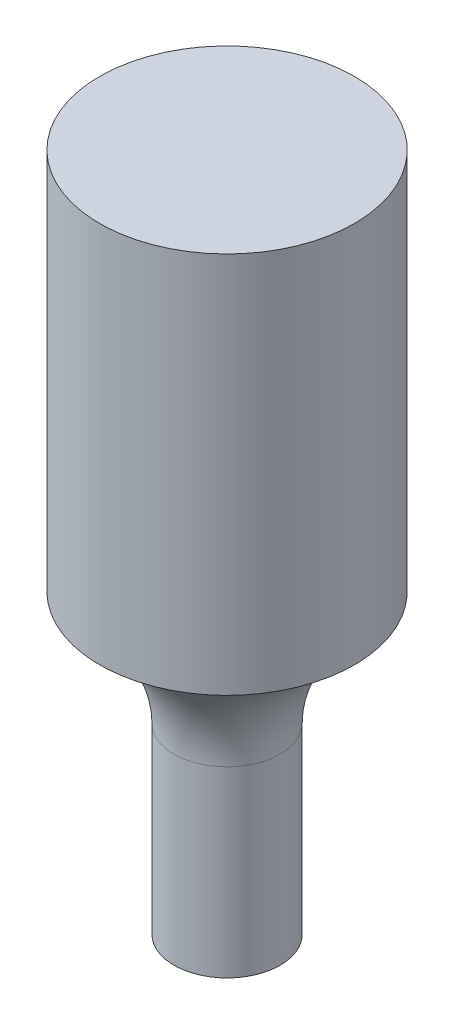
ISO-10303-21;
HEADER;
FILE_DESCRIPTION(('STEP AP214'),'2;1');
FILE_NAME('part.step','',(''),(''),'','','');
FILE_SCHEMA(('AUTOMOTIVE_DESIGN { 1 0 10303 214 1 1 1 1 }'));
ENDSEC;
DATA;
#1=APPLICATION_CONTEXT('core data for automotive mechanical design processes');
#2=APPLICATION_PROTOCOL_DEFINITION('international standard','automotive_design',2000,#1);
#3=PRODUCT_CONTEXT('',#1,'mechanical');
#4=PRODUCT('Part','Part','',(#3));
#5=PRODUCT_RELATED_PRODUCT_CATEGORY('part','',(#4));
#6=PRODUCT_DEFINITION_FORMATION('','',#4);
#7=PRODUCT_DEFINITION_CONTEXT('part definition',#1,'design');
#8=PRODUCT_DEFINITION('design','',#6,#7);
#9=PRODUCT_DEFINITION_SHAPE('','',#8);
#10=(LENGTH_UNIT() NAMED_UNIT(*) SI_UNIT(.MILLI.,.METRE.));
#11=(NAMED_UNIT(*) PLANE_ANGLE_UNIT() SI_UNIT($,.RADIAN.));
#12=(NAMED_UNIT(*) SI_UNIT($,.STERADIAN.) SOLID_ANGLE_UNIT());
#13=UNCERTAINTY_MEASURE_WITH_UNIT(LENGTH_MEASURE(1.E-05),#10,'distance_accuracy_value','');
#14=(GEOMETRIC_REPRESENTATION_CONTEXT(3) GLOBAL_UNCERTAINTY_ASSIGNED_CONTEXT((#13)) GLOBAL_UNIT_ASSIGNED_CONTEXT((#10,
#11,#12)) REPRESENTATION_CONTEXT('',''));
#15=CARTESIAN_POINT('',(0.,0.,0.));
#16=DIRECTION('',(0.,0.,1.));
#17=DIRECTION('',(1.,0.,0.));
#18=AXIS2_PLACEMENT_3D('',#15,#16,#17);
#19=CARTESIAN_POINT('',(0.,0.,0.));
#20=DIRECTION('',(0.,1.,0.));
#21=DIRECTION('',(0.,0.,1.));
#22=AXIS2_PLACEMENT_3D('',#19,#20,#21);
#23=PLANE('',#22);
#24=CARTESIAN_POINT('',(0.,0.,0.));
#25=DIRECTION('',(0.,-1.,0.));
#26=DIRECTION('',(0.,0.,-1.));
#27=AXIS2_PLACEMENT_3D('',#24,#25,#26);
#28=CIRCLE('',#27,2.5);
#29=CARTESIAN_POINT('',(0.,0.,-2.5));
#30=VERTEX_POINT('',#29);
#31=EDGE_CURVE('E10',#30,#30,#28,.T.);
#32=ORIENTED_EDGE('',*,*,#31,.T.);
#33=EDGE_LOOP('',(#32));
#34=FACE_BOUND('',#33,.T.);
#35=ADVANCED_FACE('F40',(#34),#23,.F.);
#36=CARTESIAN_POINT('',(0.,0.,0.));
#37=DIRECTION('',(0.,-1.,0.));
#38=DIRECTION('',(0.,0.,-1.));
#39=AXIS2_PLACEMENT_3D('',#36,#37,#38);
#40=CYLINDRICAL_SURFACE('',#39,2.5);
#41=ORIENTED_EDGE('',*,*,#31,.F.);
#42=EDGE_LOOP('',(#41));
#43=FACE_BOUND('',#42,.T.);
#44=CARTESIAN_POINT('',(0.,8.61019480871526,0.));
#45=DIRECTION('',(0.,-1.,0.));
#46=DIRECTION('',(0.,0.,-1.));
#47=AXIS2_PLACEMENT_3D('',#44,#45,#46);
#48=CIRCLE('',#47,2.5);
#49=CARTESIAN_POINT('',(0.,8.61019480871526,-2.5));
#50=VERTEX_POINT('',#49);
#51=EDGE_CURVE('E43',#50,#50,#48,.T.);
#52=ORIENTED_EDGE('',*,*,#51,.T.);
#53=EDGE_LOOP('',(#52));
#54=FACE_BOUND('',#53,.T.);
#55=ADVANCED_FACE('F69',(#43,#54),#40,.T.);
#56=CARTESIAN_POINT('',(0.,8.61019480871526,0.));
#57=DIRECTION('',(0.,-1.,0.));
#58=DIRECTION('',(0.,0.,-1.));
#59=AXIS2_PLACEMENT_3D('',#56,#57,#58);
#60=TOROIDAL_SURFACE('',#59,8.4,5.9);
#61=ORIENTED_EDGE('',*,*,#51,.F.);
#62=EDGE_LOOP('',(#61));
#63=FACE_BOUND('',#62,.T.);
#64=CARTESIAN_POINT('',(0.,14.,0.));
#65=DIRECTION('',(0.,-1.,0.));
#66=DIRECTION('',(0.,0.,-1.));
#67=AXIS2_PLACEMENT_3D('',#64,#65,#66);
#68=CIRCLE('',#67,6.);
#69=CARTESIAN_POINT('',(0.,14.,-6.));
#70=VERTEX_POINT('',#69);
#71=EDGE_CURVE('E50',#70,#70,#68,.T.);
#72=ORIENTED_EDGE('',*,*,#71,.T.);
#73=EDGE_LOOP('',(#72));
#74=FACE_BOUND('',#73,.T.);
#75=ADVANCED_FACE('F64',(#63,#74),#60,.F.);
#76=CARTESIAN_POINT('',(0.,0.,0.));
#77=DIRECTION('',(0.,-1.,0.));
#78=DIRECTION('',(0.,0.,-1.));
#79=AXIS2_PLACEMENT_3D('',#76,#77,#78);
#80=CYLINDRICAL_SURFACE('',#79,6.);
#81=ORIENTED_EDGE('',*,*,#71,.F.);
#82=EDGE_LOOP('',(#81));
#83=FACE_BOUND('',#82,.T.);
#84=CARTESIAN_POINT('',(0.,32.,0.));
#85=DIRECTION('',(0.,-1.,0.));
#86=DIRECTION('',(0.,0.,-1.));
#87=AXIS2_PLACEMENT_3D('',#84,#85,#86);
#88=CIRCLE('',#87,6.);
#89=CARTESIAN_POINT('',(0.,32.,-6.));
#90=VERTEX_POINT('',#89);
#91=EDGE_CURVE('E51',#90,#90,#88,.T.);
#92=ORIENTED_EDGE('',*,*,#91,.T.);
#93=EDGE_LOOP('',(#92));
#94=FACE_BOUND('',#93,.T.);
#95=ADVANCED_FACE('F60',(#83,#94),#80,.T.);
#96=CARTESIAN_POINT('',(0.,32.,0.));
#97=DIRECTION('',(0.,-1.,0.));
#98=DIRECTION('',(0.,0.,-1.));
#99=AXIS2_PLACEMENT_3D('',#96,#97,#98);
#100=PLANE('',#99);
#101=ORIENTED_EDGE('',*,*,#91,.F.);
#102=EDGE_LOOP('',(#101));
#103=FACE_BOUND('',#102,.T.);
#104=ADVANCED_FACE('F56',(#103),#100,.F.);
#105=CLOSED_SHELL('',(#35,#55,#75,#95,#104));
#106=MANIFOLD_SOLID_BREP('B2',#105);
#107=ADVANCED_BREP_SHAPE_REPRESENTATION('',(#18,#106),#14);
#108=SHAPE_DEFINITION_REPRESENTATION(#9,#107);
ENDSEC;
END-ISO-10303-21;
